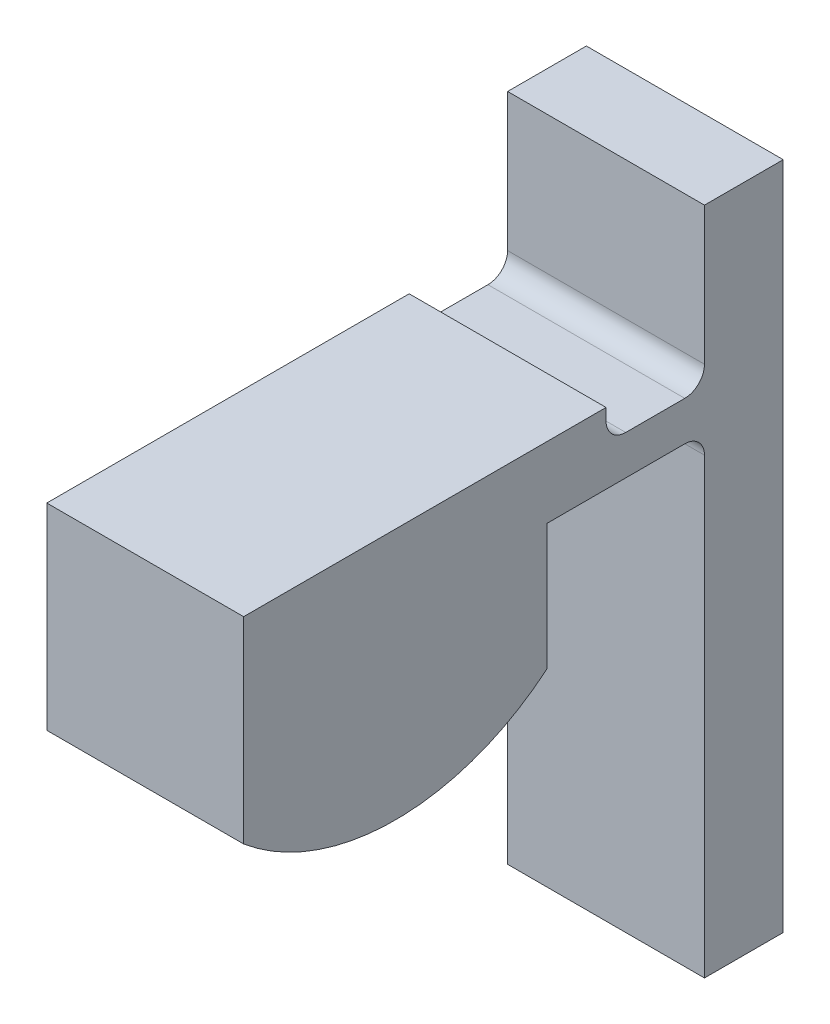
ISO-10303-21;
HEADER;
FILE_DESCRIPTION(('STEP AP214'),'2;1');
FILE_NAME('part.step','',(''),(''),'','','');
FILE_SCHEMA(('AUTOMOTIVE_DESIGN { 1 0 10303 214 1 1 1 1 }'));
ENDSEC;
DATA;
#1=APPLICATION_CONTEXT('core data for automotive mechanical design processes');
#2=APPLICATION_PROTOCOL_DEFINITION('international standard','automotive_design',2000,#1);
#3=PRODUCT_CONTEXT('',#1,'mechanical');
#4=PRODUCT('Part','Part','',(#3));
#5=PRODUCT_RELATED_PRODUCT_CATEGORY('part','',(#4));
#6=PRODUCT_DEFINITION_FORMATION('','',#4);
#7=PRODUCT_DEFINITION_CONTEXT('part definition',#1,'design');
#8=PRODUCT_DEFINITION('design','',#6,#7);
#9=PRODUCT_DEFINITION_SHAPE('','',#8);
#10=(LENGTH_UNIT() NAMED_UNIT(*) SI_UNIT(.MILLI.,.METRE.));
#11=(NAMED_UNIT(*) PLANE_ANGLE_UNIT() SI_UNIT($,.RADIAN.));
#12=(NAMED_UNIT(*) SI_UNIT($,.STERADIAN.) SOLID_ANGLE_UNIT());
#13=UNCERTAINTY_MEASURE_WITH_UNIT(LENGTH_MEASURE(1.E-05),#10,'distance_accuracy_value','');
#14=(GEOMETRIC_REPRESENTATION_CONTEXT(3) GLOBAL_UNCERTAINTY_ASSIGNED_CONTEXT((#13)) GLOBAL_UNIT_ASSIGNED_CONTEXT((#10,
#11,#12)) REPRESENTATION_CONTEXT('',''));
#15=CARTESIAN_POINT('',(0.,0.,0.));
#16=DIRECTION('',(0.,0.,1.));
#17=DIRECTION('',(1.,0.,0.));
#18=AXIS2_PLACEMENT_3D('',#15,#16,#17);
#19=CARTESIAN_POINT('',(25.,85.,10.));
#20=DIRECTION('',(0.,0.,-1.));
#21=DIRECTION('',(0.,1.,0.));
#22=AXIS2_PLACEMENT_3D('',#19,#20,#21);
#23=PLANE('',#22);
#24=DIRECTION('',(0.,-1.,0.));
#25=VECTOR('',#24,1.);
#26=CARTESIAN_POINT('',(25.,85.,10.));
#27=LINE('',#26,#25);
#28=CARTESIAN_POINT('',(25.,30.,10.));
#29=VERTEX_POINT('',#28);
#30=CARTESIAN_POINT('',(25.,-85.,9.99999999999999));
#31=VERTEX_POINT('',#30);
#32=EDGE_CURVE('E221',#29,#31,#27,.T.);
#33=ORIENTED_EDGE('',*,*,#32,.F.);
#34=DIRECTION('',(1.,0.,0.));
#35=VECTOR('',#34,1.);
#36=CARTESIAN_POINT('',(25.,30.,10.));
#37=LINE('',#36,#35);
#38=CARTESIAN_POINT('',(-25.,30.,10.));
#39=VERTEX_POINT('',#38);
#40=EDGE_CURVE('E251',#29,#39,#37,.F.);
#41=ORIENTED_EDGE('',*,*,#40,.T.);
#42=DIRECTION('',(0.,-1.,0.));
#43=VECTOR('',#42,1.);
#44=CARTESIAN_POINT('',(-25.,85.,10.));
#45=LINE('',#44,#43);
#46=CARTESIAN_POINT('',(-25.,-85.,9.99999999999999));
#47=VERTEX_POINT('',#46);
#48=EDGE_CURVE('E231',#39,#47,#45,.T.);
#49=ORIENTED_EDGE('',*,*,#48,.T.);
#50=DIRECTION('',(-1.,0.,0.));
#51=VECTOR('',#50,1.);
#52=CARTESIAN_POINT('',(25.,-85.,9.99999999999999));
#53=LINE('',#52,#51);
#54=EDGE_CURVE('E242',#31,#47,#53,.T.);
#55=ORIENTED_EDGE('',*,*,#54,.F.);
#56=EDGE_LOOP('',(#33,#41,#49,#55));
#57=FACE_BOUND('',#56,.T.);
#58=ADVANCED_FACE('F39',(#57),#23,.F.);
#59=CARTESIAN_POINT('',(25.,85.,-9.99999999999998));
#60=DIRECTION('',(0.,0.,1.));
#61=DIRECTION('',(0.,-1.,0.));
#62=AXIS2_PLACEMENT_3D('',#59,#60,#61);
#63=PLANE('',#62);
#64=DIRECTION('',(0.,1.,0.));
#65=VECTOR('',#64,1.);
#66=CARTESIAN_POINT('',(-25.,85.,-9.99999999999998));
#67=LINE('',#66,#65);
#68=CARTESIAN_POINT('',(-25.,-85.,-10.));
#69=VERTEX_POINT('',#68);
#70=CARTESIAN_POINT('',(-25.,85.,-9.99999999999998));
#71=VERTEX_POINT('',#70);
#72=EDGE_CURVE('E215',#69,#71,#67,.T.);
#73=ORIENTED_EDGE('',*,*,#72,.T.);
#74=DIRECTION('',(-1.,0.,0.));
#75=VECTOR('',#74,1.);
#76=CARTESIAN_POINT('',(25.,85.,-9.99999999999998));
#77=LINE('',#76,#75);
#78=CARTESIAN_POINT('',(25.,85.,-9.99999999999998));
#79=VERTEX_POINT('',#78);
#80=EDGE_CURVE('E250',#79,#71,#77,.T.);
#81=ORIENTED_EDGE('',*,*,#80,.F.);
#82=DIRECTION('',(0.,1.,0.));
#83=VECTOR('',#82,1.);
#84=CARTESIAN_POINT('',(25.,85.,-9.99999999999998));
#85=LINE('',#84,#83);
#86=CARTESIAN_POINT('',(25.,-85.,-10.));
#87=VERTEX_POINT('',#86);
#88=EDGE_CURVE('E217',#87,#79,#85,.T.);
#89=ORIENTED_EDGE('',*,*,#88,.F.);
#90=DIRECTION('',(-1.,0.,0.));
#91=VECTOR('',#90,1.);
#92=CARTESIAN_POINT('',(25.,-85.,-10.));
#93=LINE('',#92,#91);
#94=EDGE_CURVE('E226',#87,#69,#93,.T.);
#95=ORIENTED_EDGE('',*,*,#94,.T.);
#96=EDGE_LOOP('',(#73,#81,#89,#95));
#97=FACE_BOUND('',#96,.T.);
#98=ADVANCED_FACE('F285',(#97),#63,.F.);
#99=CARTESIAN_POINT('',(25.,85.,10.));
#100=DIRECTION('',(0.,-1.,0.));
#101=DIRECTION('',(0.,0.,-1.));
#102=AXIS2_PLACEMENT_3D('',#99,#100,#101);
#103=PLANE('',#102);
#104=DIRECTION('',(0.,0.,1.));
#105=VECTOR('',#104,1.);
#106=CARTESIAN_POINT('',(-25.,85.,10.));
#107=LINE('',#106,#105);
#108=CARTESIAN_POINT('',(-25.,85.,10.));
#109=VERTEX_POINT('',#108);
#110=EDGE_CURVE('E235',#71,#109,#107,.T.);
#111=ORIENTED_EDGE('',*,*,#110,.T.);
#112=DIRECTION('',(-1.,0.,0.));
#113=VECTOR('',#112,1.);
#114=CARTESIAN_POINT('',(25.,85.,10.));
#115=LINE('',#114,#113);
#116=CARTESIAN_POINT('',(25.,85.,10.));
#117=VERTEX_POINT('',#116);
#118=EDGE_CURVE('E241',#117,#109,#115,.T.);
#119=ORIENTED_EDGE('',*,*,#118,.F.);
#120=DIRECTION('',(0.,0.,1.));
#121=VECTOR('',#120,1.);
#122=CARTESIAN_POINT('',(25.,85.,10.));
#123=LINE('',#122,#121);
#124=EDGE_CURVE('E222',#79,#117,#123,.T.);
#125=ORIENTED_EDGE('',*,*,#124,.F.);
#126=ORIENTED_EDGE('',*,*,#80,.T.);
#127=EDGE_LOOP('',(#111,#119,#125,#126));
#128=FACE_BOUND('',#127,.T.);
#129=ADVANCED_FACE('F283',(#128),#103,.F.);
#130=CARTESIAN_POINT('',(-25.,50.,10.));
#131=VERTEX_POINT('',#130);
#132=EDGE_CURVE('E233',#109,#131,#45,.T.);
#133=ORIENTED_EDGE('',*,*,#132,.T.);
#134=DIRECTION('',(1.,0.,0.));
#135=VECTOR('',#134,1.);
#136=CARTESIAN_POINT('',(25.,50.,10.));
#137=LINE('',#136,#135);
#138=CARTESIAN_POINT('',(25.,50.,10.));
#139=VERTEX_POINT('',#138);
#140=EDGE_CURVE('E254',#131,#139,#137,.T.);
#141=ORIENTED_EDGE('',*,*,#140,.T.);
#142=EDGE_CURVE('E223',#117,#139,#27,.T.);
#143=ORIENTED_EDGE('',*,*,#142,.F.);
#144=ORIENTED_EDGE('',*,*,#118,.T.);
#145=EDGE_LOOP('',(#133,#141,#143,#144));
#146=FACE_BOUND('',#145,.T.);
#147=ADVANCED_FACE('F286',(#146),#23,.F.);
#148=CARTESIAN_POINT('',(25.,-85.,9.99999999999999));
#149=DIRECTION('',(0.,1.,0.));
#150=DIRECTION('',(0.,0.,1.));
#151=AXIS2_PLACEMENT_3D('',#148,#149,#150);
#152=PLANE('',#151);
#153=DIRECTION('',(0.,0.,-1.));
#154=VECTOR('',#153,1.);
#155=CARTESIAN_POINT('',(-25.,-85.,9.99999999999999));
#156=LINE('',#155,#154);
#157=EDGE_CURVE('E225',#47,#69,#156,.T.);
#158=ORIENTED_EDGE('',*,*,#157,.T.);
#159=ORIENTED_EDGE('',*,*,#94,.F.);
#160=DIRECTION('',(0.,0.,-1.));
#161=VECTOR('',#160,1.);
#162=CARTESIAN_POINT('',(25.,-85.,9.99999999999999));
#163=LINE('',#162,#161);
#164=EDGE_CURVE('E229',#31,#87,#163,.T.);
#165=ORIENTED_EDGE('',*,*,#164,.F.);
#166=ORIENTED_EDGE('',*,*,#54,.T.);
#167=EDGE_LOOP('',(#158,#159,#165,#166));
#168=FACE_BOUND('',#167,.T.);
#169=ADVANCED_FACE('F279',(#168),#152,.F.);
#170=CARTESIAN_POINT('',(25.,0.,0.));
#171=DIRECTION('',(1.,0.,0.));
#172=DIRECTION('',(0.,0.,-1.));
#173=AXIS2_PLACEMENT_3D('',#170,#171,#172);
#174=PLANE('',#173);
#175=ORIENTED_EDGE('',*,*,#88,.T.);
#176=ORIENTED_EDGE('',*,*,#124,.T.);
#177=ORIENTED_EDGE('',*,*,#142,.T.);
#178=CARTESIAN_POINT('',(25.,50.,15.));
#179=DIRECTION('',(1.,0.,0.));
#180=DIRECTION('',(0.,0.,-1.));
#181=AXIS2_PLACEMENT_3D('',#178,#179,#180);
#182=CIRCLE('',#181,5.);
#183=CARTESIAN_POINT('',(25.,45.,15.));
#184=VERTEX_POINT('',#183);
#185=EDGE_CURVE('E50',#139,#184,#182,.F.);
#186=ORIENTED_EDGE('',*,*,#185,.T.);
#187=DIRECTION('',(0.,0.,-1.));
#188=VECTOR('',#187,1.);
#189=CARTESIAN_POINT('',(25.,45.,30.));
#190=LINE('',#189,#188);
#191=CARTESIAN_POINT('',(25.,45.,30.));
#192=VERTEX_POINT('',#191);
#193=EDGE_CURVE('E201',#192,#184,#190,.T.);
#194=ORIENTED_EDGE('',*,*,#193,.F.);
#195=CARTESIAN_POINT('',(25.,50.,30.));
#196=DIRECTION('',(-1.,0.,0.));
#197=DIRECTION('',(0.,0.,1.));
#198=AXIS2_PLACEMENT_3D('',#195,#196,#197);
#199=CIRCLE('',#198,5.);
#200=CARTESIAN_POINT('',(25.,50.,35.));
#201=VERTEX_POINT('',#200);
#202=EDGE_CURVE('E202',#192,#201,#199,.T.);
#203=ORIENTED_EDGE('',*,*,#202,.T.);
#204=DIRECTION('',(0.,1.,0.));
#205=VECTOR('',#204,1.);
#206=CARTESIAN_POINT('',(25.,50.,35.));
#207=LINE('',#206,#205);
#208=CARTESIAN_POINT('',(25.,53.,35.));
#209=VERTEX_POINT('',#208);
#210=EDGE_CURVE('E190',#201,#209,#207,.T.);
#211=ORIENTED_EDGE('',*,*,#210,.T.);
#212=DIRECTION('',(0.,0.,1.));
#213=VECTOR('',#212,1.);
#214=CARTESIAN_POINT('',(25.,53.,35.));
#215=LINE('',#214,#213);
#216=CARTESIAN_POINT('',(25.,53.,127.045441137033));
#217=VERTEX_POINT('',#216);
#218=EDGE_CURVE('E181',#209,#217,#215,.T.);
#219=ORIENTED_EDGE('',*,*,#218,.T.);
#220=DIRECTION('',(0.,-1.,0.));
#221=VECTOR('',#220,1.);
#222=CARTESIAN_POINT('',(25.,2.99999999999999,127.045441137033));
#223=LINE('',#222,#221);
#224=CARTESIAN_POINT('',(25.,2.99999999999999,127.045441137033));
#225=VERTEX_POINT('',#224);
#226=EDGE_CURVE('E175',#217,#225,#223,.T.);
#227=ORIENTED_EDGE('',*,*,#226,.T.);
#228=CARTESIAN_POINT('',(25.,49.,88.5227205685165));
#229=DIRECTION('',(1.,0.,0.));
#230=DIRECTION('',(0.,0.,-1.));
#231=AXIS2_PLACEMENT_3D('',#228,#229,#230);
#232=CIRCLE('',#231,60.);
#233=CARTESIAN_POINT('',(25.,3.,50.));
#234=VERTEX_POINT('',#233);
#235=EDGE_CURVE('E176',#225,#234,#232,.T.);
#236=ORIENTED_EDGE('',*,*,#235,.T.);
#237=DIRECTION('',(0.,1.,0.));
#238=VECTOR('',#237,1.);
#239=CARTESIAN_POINT('',(25.,53.,50.));
#240=LINE('',#239,#238);
#241=CARTESIAN_POINT('',(25.,35.,50.));
#242=VERTEX_POINT('',#241);
#243=EDGE_CURVE('E155',#234,#242,#240,.T.);
#244=ORIENTED_EDGE('',*,*,#243,.T.);
#245=DIRECTION('',(0.,0.,-1.));
#246=VECTOR('',#245,1.);
#247=CARTESIAN_POINT('',(25.,35.,50.));
#248=LINE('',#247,#246);
#249=CARTESIAN_POINT('',(25.,35.,15.));
#250=VERTEX_POINT('',#249);
#251=EDGE_CURVE('E199',#242,#250,#248,.T.);
#252=ORIENTED_EDGE('',*,*,#251,.T.);
#253=CARTESIAN_POINT('',(25.,30.,15.));
#254=DIRECTION('',(1.,0.,0.));
#255=DIRECTION('',(0.,0.,-1.));
#256=AXIS2_PLACEMENT_3D('',#253,#254,#255);
#257=CIRCLE('',#256,5.);
#258=EDGE_CURVE('E259',#250,#29,#257,.F.);
#259=ORIENTED_EDGE('',*,*,#258,.T.);
#260=ORIENTED_EDGE('',*,*,#32,.T.);
#261=ORIENTED_EDGE('',*,*,#164,.T.);
#262=EDGE_LOOP('',(#175,#176,#177,#186,#194,#203,#211,#219,#227,#236,#244,#252,#259,#260,#261));
#263=FACE_BOUND('',#262,.T.);
#264=ADVANCED_FACE('F275',(#263),#174,.T.);
#265=CARTESIAN_POINT('',(-25.,0.,0.));
#266=DIRECTION('',(1.,0.,0.));
#267=DIRECTION('',(0.,0.,-1.));
#268=AXIS2_PLACEMENT_3D('',#265,#266,#267);
#269=PLANE('',#268);
#270=ORIENTED_EDGE('',*,*,#72,.F.);
#271=ORIENTED_EDGE('',*,*,#157,.F.);
#272=ORIENTED_EDGE('',*,*,#48,.F.);
#273=CARTESIAN_POINT('',(-25.,30.,15.));
#274=DIRECTION('',(1.,0.,0.));
#275=DIRECTION('',(0.,0.,-1.));
#276=AXIS2_PLACEMENT_3D('',#273,#274,#275);
#277=CIRCLE('',#276,5.);
#278=CARTESIAN_POINT('',(-25.,35.,15.));
#279=VERTEX_POINT('',#278);
#280=EDGE_CURVE('E261',#39,#279,#277,.T.);
#281=ORIENTED_EDGE('',*,*,#280,.T.);
#282=DIRECTION('',(0.,0.,-1.));
#283=VECTOR('',#282,1.);
#284=CARTESIAN_POINT('',(-25.,35.,50.));
#285=LINE('',#284,#283);
#286=CARTESIAN_POINT('',(-25.,35.,50.));
#287=VERTEX_POINT('',#286);
#288=EDGE_CURVE('E166',#287,#279,#285,.T.);
#289=ORIENTED_EDGE('',*,*,#288,.F.);
#290=DIRECTION('',(0.,1.,0.));
#291=VECTOR('',#290,1.);
#292=CARTESIAN_POINT('',(-25.,53.,50.));
#293=LINE('',#292,#291);
#294=CARTESIAN_POINT('',(-25.,3.,50.));
#295=VERTEX_POINT('',#294);
#296=EDGE_CURVE('E147',#295,#287,#293,.T.);
#297=ORIENTED_EDGE('',*,*,#296,.F.);
#298=CARTESIAN_POINT('',(-25.,49.,88.5227205685165));
#299=DIRECTION('',(1.,0.,0.));
#300=DIRECTION('',(0.,0.,-1.));
#301=AXIS2_PLACEMENT_3D('',#298,#299,#300);
#302=CIRCLE('',#301,60.);
#303=CARTESIAN_POINT('',(-25.,2.99999999999999,127.045441137033));
#304=VERTEX_POINT('',#303);
#305=EDGE_CURVE('E167',#304,#295,#302,.T.);
#306=ORIENTED_EDGE('',*,*,#305,.F.);
#307=DIRECTION('',(0.,-1.,0.));
#308=VECTOR('',#307,1.);
#309=CARTESIAN_POINT('',(-25.,2.99999999999999,127.045441137033));
#310=LINE('',#309,#308);
#311=CARTESIAN_POINT('',(-25.,53.,127.045441137033));
#312=VERTEX_POINT('',#311);
#313=EDGE_CURVE('E158',#312,#304,#310,.T.);
#314=ORIENTED_EDGE('',*,*,#313,.F.);
#315=DIRECTION('',(0.,0.,1.));
#316=VECTOR('',#315,1.);
#317=CARTESIAN_POINT('',(-25.,53.,35.));
#318=LINE('',#317,#316);
#319=CARTESIAN_POINT('',(-25.,53.,35.));
#320=VERTEX_POINT('',#319);
#321=EDGE_CURVE('E187',#320,#312,#318,.T.);
#322=ORIENTED_EDGE('',*,*,#321,.F.);
#323=DIRECTION('',(0.,1.,0.));
#324=VECTOR('',#323,1.);
#325=CARTESIAN_POINT('',(-25.,50.,35.));
#326=LINE('',#325,#324);
#327=CARTESIAN_POINT('',(-25.,50.,35.));
#328=VERTEX_POINT('',#327);
#329=EDGE_CURVE('E193',#328,#320,#326,.T.);
#330=ORIENTED_EDGE('',*,*,#329,.F.);
#331=CARTESIAN_POINT('',(-25.,50.,30.));
#332=DIRECTION('',(-1.,0.,0.));
#333=DIRECTION('',(0.,0.,1.));
#334=AXIS2_PLACEMENT_3D('',#331,#332,#333);
#335=CIRCLE('',#334,5.);
#336=CARTESIAN_POINT('',(-25.,45.,30.));
#337=VERTEX_POINT('',#336);
#338=EDGE_CURVE('E195',#337,#328,#335,.T.);
#339=ORIENTED_EDGE('',*,*,#338,.F.);
#340=DIRECTION('',(0.,0.,-1.));
#341=VECTOR('',#340,1.);
#342=CARTESIAN_POINT('',(-25.,45.,30.));
#343=LINE('',#342,#341);
#344=CARTESIAN_POINT('',(-25.,45.,15.));
#345=VERTEX_POINT('',#344);
#346=EDGE_CURVE('E188',#337,#345,#343,.T.);
#347=ORIENTED_EDGE('',*,*,#346,.T.);
#348=CARTESIAN_POINT('',(-25.,50.,15.));
#349=DIRECTION('',(1.,0.,0.));
#350=DIRECTION('',(0.,0.,-1.));
#351=AXIS2_PLACEMENT_3D('',#348,#349,#350);
#352=CIRCLE('',#351,5.);
#353=EDGE_CURVE('E11',#345,#131,#352,.T.);
#354=ORIENTED_EDGE('',*,*,#353,.T.);
#355=ORIENTED_EDGE('',*,*,#132,.F.);
#356=ORIENTED_EDGE('',*,*,#110,.F.);
#357=EDGE_LOOP('',(#270,#271,#272,#281,#289,#297,#306,#314,#322,#330,#339,#347,#354,#355,#356));
#358=FACE_BOUND('',#357,.T.);
#359=ADVANCED_FACE('F163',(#358),#269,.F.);
#360=CARTESIAN_POINT('',(-25.,53.,35.));
#361=DIRECTION('',(0.,1.,0.));
#362=DIRECTION('',(0.,0.,1.));
#363=AXIS2_PLACEMENT_3D('',#360,#361,#362);
#364=PLANE('',#363);
#365=ORIENTED_EDGE('',*,*,#218,.F.);
#366=DIRECTION('',(1.,0.,0.));
#367=VECTOR('',#366,1.);
#368=CARTESIAN_POINT('',(-25.,53.,35.));
#369=LINE('',#368,#367);
#370=EDGE_CURVE('E209',#320,#209,#369,.T.);
#371=ORIENTED_EDGE('',*,*,#370,.F.);
#372=ORIENTED_EDGE('',*,*,#321,.T.);
#373=DIRECTION('',(1.,0.,0.));
#374=VECTOR('',#373,1.);
#375=CARTESIAN_POINT('',(-25.,53.,127.045441137033));
#376=LINE('',#375,#374);
#377=EDGE_CURVE('E160',#312,#217,#376,.T.);
#378=ORIENTED_EDGE('',*,*,#377,.T.);
#379=EDGE_LOOP('',(#365,#371,#372,#378));
#380=FACE_BOUND('',#379,.T.);
#381=ADVANCED_FACE('F308',(#380),#364,.T.);
#382=CARTESIAN_POINT('',(-25.,50.,35.));
#383=DIRECTION('',(0.,0.,-1.));
#384=DIRECTION('',(-1.,0.,0.));
#385=AXIS2_PLACEMENT_3D('',#382,#383,#384);
#386=PLANE('',#385);
#387=ORIENTED_EDGE('',*,*,#210,.F.);
#388=DIRECTION('',(1.,0.,0.));
#389=VECTOR('',#388,1.);
#390=CARTESIAN_POINT('',(-25.,50.,35.));
#391=LINE('',#390,#389);
#392=EDGE_CURVE('E213',#328,#201,#391,.T.);
#393=ORIENTED_EDGE('',*,*,#392,.F.);
#394=ORIENTED_EDGE('',*,*,#329,.T.);
#395=ORIENTED_EDGE('',*,*,#370,.T.);
#396=EDGE_LOOP('',(#387,#393,#394,#395));
#397=FACE_BOUND('',#396,.T.);
#398=ADVANCED_FACE('F302',(#397),#386,.T.);
#399=CARTESIAN_POINT('',(-25.,50.,30.));
#400=DIRECTION('',(1.,0.,0.));
#401=DIRECTION('',(0.,0.,-1.));
#402=AXIS2_PLACEMENT_3D('',#399,#400,#401);
#403=CYLINDRICAL_SURFACE('',#402,5.);
#404=ORIENTED_EDGE('',*,*,#202,.F.);
#405=DIRECTION('',(1.,0.,0.));
#406=VECTOR('',#405,1.);
#407=CARTESIAN_POINT('',(-25.,45.,30.));
#408=LINE('',#407,#406);
#409=EDGE_CURVE('E214',#337,#192,#408,.T.);
#410=ORIENTED_EDGE('',*,*,#409,.F.);
#411=ORIENTED_EDGE('',*,*,#338,.T.);
#412=ORIENTED_EDGE('',*,*,#392,.T.);
#413=EDGE_LOOP('',(#404,#410,#411,#412));
#414=FACE_BOUND('',#413,.T.);
#415=ADVANCED_FACE('F296',(#414),#403,.F.);
#416=CARTESIAN_POINT('',(-25.,45.,30.));
#417=DIRECTION('',(0.,-1.,0.));
#418=DIRECTION('',(0.,0.,-1.));
#419=AXIS2_PLACEMENT_3D('',#416,#417,#418);
#420=PLANE('',#419);
#421=ORIENTED_EDGE('',*,*,#193,.T.);
#422=DIRECTION('',(1.,0.,0.));
#423=VECTOR('',#422,1.);
#424=CARTESIAN_POINT('',(-25.,45.,15.));
#425=LINE('',#424,#423);
#426=EDGE_CURVE('E53',#184,#345,#425,.F.);
#427=ORIENTED_EDGE('',*,*,#426,.T.);
#428=ORIENTED_EDGE('',*,*,#346,.F.);
#429=ORIENTED_EDGE('',*,*,#409,.T.);
#430=EDGE_LOOP('',(#421,#427,#428,#429));
#431=FACE_BOUND('',#430,.T.);
#432=ADVANCED_FACE('F293',(#431),#420,.F.);
#433=CARTESIAN_POINT('',(-25.,35.,50.));
#434=DIRECTION('',(0.,-1.,0.));
#435=DIRECTION('',(0.,0.,-1.));
#436=AXIS2_PLACEMENT_3D('',#433,#434,#435);
#437=PLANE('',#436);
#438=ORIENTED_EDGE('',*,*,#288,.T.);
#439=DIRECTION('',(1.,0.,0.));
#440=VECTOR('',#439,1.);
#441=CARTESIAN_POINT('',(-25.,35.,15.));
#442=LINE('',#441,#440);
#443=EDGE_CURVE('E248',#279,#250,#442,.T.);
#444=ORIENTED_EDGE('',*,*,#443,.T.);
#445=ORIENTED_EDGE('',*,*,#251,.F.);
#446=DIRECTION('',(1.,0.,0.));
#447=VECTOR('',#446,1.);
#448=CARTESIAN_POINT('',(-25.,35.,50.));
#449=LINE('',#448,#447);
#450=EDGE_CURVE('E196',#287,#242,#449,.T.);
#451=ORIENTED_EDGE('',*,*,#450,.F.);
#452=EDGE_LOOP('',(#438,#444,#445,#451));
#453=FACE_BOUND('',#452,.T.);
#454=ADVANCED_FACE('F267',(#453),#437,.T.);
#455=CARTESIAN_POINT('',(-25.,30.,15.));
#456=DIRECTION('',(1.,0.,0.));
#457=DIRECTION('',(0.,0.,-1.));
#458=AXIS2_PLACEMENT_3D('',#455,#456,#457);
#459=CYLINDRICAL_SURFACE('',#458,5.);
#460=ORIENTED_EDGE('',*,*,#280,.F.);
#461=ORIENTED_EDGE('',*,*,#40,.F.);
#462=ORIENTED_EDGE('',*,*,#258,.F.);
#463=ORIENTED_EDGE('',*,*,#443,.F.);
#464=EDGE_LOOP('',(#460,#461,#462,#463));
#465=FACE_BOUND('',#464,.T.);
#466=ADVANCED_FACE('F269',(#465),#459,.F.);
#467=CARTESIAN_POINT('',(25.,50.,15.));
#468=DIRECTION('',(-1.,0.,0.));
#469=DIRECTION('',(0.,0.,1.));
#470=AXIS2_PLACEMENT_3D('',#467,#468,#469);
#471=CYLINDRICAL_SURFACE('',#470,5.);
#472=ORIENTED_EDGE('',*,*,#353,.F.);
#473=ORIENTED_EDGE('',*,*,#426,.F.);
#474=ORIENTED_EDGE('',*,*,#185,.F.);
#475=ORIENTED_EDGE('',*,*,#140,.F.);
#476=EDGE_LOOP('',(#472,#473,#474,#475));
#477=FACE_BOUND('',#476,.T.);
#478=ADVANCED_FACE('F41',(#477),#471,.F.);
#479=CARTESIAN_POINT('',(-25.,49.,88.5227205685165));
#480=DIRECTION('',(1.,0.,0.));
#481=DIRECTION('',(0.,0.,-1.));
#482=AXIS2_PLACEMENT_3D('',#479,#480,#481);
#483=CYLINDRICAL_SURFACE('',#482,60.);
#484=ORIENTED_EDGE('',*,*,#235,.F.);
#485=DIRECTION('',(1.,0.,0.));
#486=VECTOR('',#485,1.);
#487=CARTESIAN_POINT('',(-25.,2.99999999999999,127.045441137033));
#488=LINE('',#487,#486);
#489=EDGE_CURVE('E174',#304,#225,#488,.T.);
#490=ORIENTED_EDGE('',*,*,#489,.F.);
#491=ORIENTED_EDGE('',*,*,#305,.T.);
#492=DIRECTION('',(1.,0.,0.));
#493=VECTOR('',#492,1.);
#494=CARTESIAN_POINT('',(-25.,3.,50.));
#495=LINE('',#494,#493);
#496=EDGE_CURVE('E148',#295,#234,#495,.T.);
#497=ORIENTED_EDGE('',*,*,#496,.T.);
#498=EDGE_LOOP('',(#484,#490,#491,#497));
#499=FACE_BOUND('',#498,.T.);
#500=ADVANCED_FACE('F172',(#499),#483,.T.);
#501=CARTESIAN_POINT('',(-25.,2.99999999999999,127.045441137033));
#502=DIRECTION('',(0.,0.,1.));
#503=DIRECTION('',(1.,0.,0.));
#504=AXIS2_PLACEMENT_3D('',#501,#502,#503);
#505=PLANE('',#504);
#506=ORIENTED_EDGE('',*,*,#226,.F.);
#507=ORIENTED_EDGE('',*,*,#377,.F.);
#508=ORIENTED_EDGE('',*,*,#313,.T.);
#509=ORIENTED_EDGE('',*,*,#489,.T.);
#510=EDGE_LOOP('',(#506,#507,#508,#509));
#511=FACE_BOUND('',#510,.T.);
#512=ADVANCED_FACE('F310',(#511),#505,.T.);
#513=CARTESIAN_POINT('',(-25.,53.,50.));
#514=DIRECTION('',(0.,0.,-1.));
#515=DIRECTION('',(0.,1.,0.));
#516=AXIS2_PLACEMENT_3D('',#513,#514,#515);
#517=PLANE('',#516);
#518=ORIENTED_EDGE('',*,*,#296,.T.);
#519=ORIENTED_EDGE('',*,*,#450,.T.);
#520=ORIENTED_EDGE('',*,*,#243,.F.);
#521=ORIENTED_EDGE('',*,*,#496,.F.);
#522=EDGE_LOOP('',(#518,#519,#520,#521));
#523=FACE_BOUND('',#522,.T.);
#524=ADVANCED_FACE('F146',(#523),#517,.T.);
#525=CLOSED_SHELL('',(#58,#98,#129,#147,#169,#264,#359,#381,#398,#415,#432,#454,#466,#478,#500,
#512,#524));
#526=MANIFOLD_SOLID_BREP('B2',#525);
#527=ADVANCED_BREP_SHAPE_REPRESENTATION('',(#18,#526),#14);
#528=SHAPE_DEFINITION_REPRESENTATION(#9,#527);
ENDSEC;
END-ISO-10303-21;
